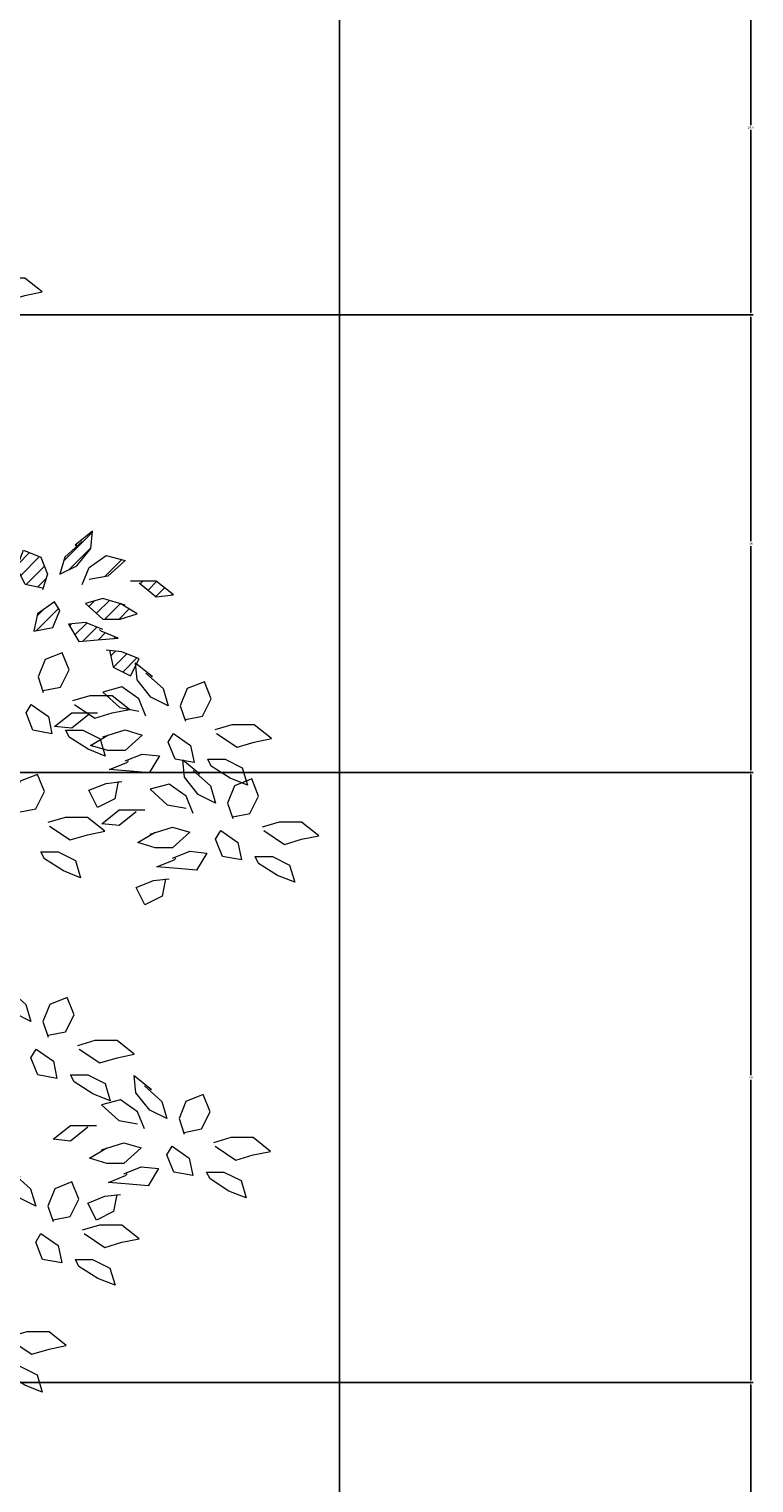
# Model space of a CAD drawing. Units: inches. Extents: x 1770 to 2988, y 1161 to 3221.
# Tile 43 of 44: x 2745 to 2802, y 2750 to 2865. Entities that reach past the tile are written whole.
import ezdxf

# ---------------------------------------------------------------- set-up
doc = ezdxf.new("R2010")
doc.units = ezdxf.units.IN
for name, color, linetype, lineweight in [('A-ANNO-DIMS', 2, 'Continuous', 18), ('A-ANNO-TTLB', 7, 'Continuous', 25), ('trees1', 250, 'Continuous', 13)]:
    doc.layers.add(name, color=color, linetype=linetype, lineweight=lineweight)
doc.styles.get("Standard").update_dxf_attribs({"font": 'arial.ttf'})
doc.dimstyles.get("Standard").update_dxf_attribs({"dimtxt": 0.18, "dimasz": 0.18, "dimexe": 0.18, "dimexo": 0.0625, "dimgap": 0.09, "dimtad": 0, "dimtih": 1, "dimtoh": 1, "dimdec": 4, "dimzin": 0, "dimdsep": 46, "dimtxsty": 'Standard', "dimcen": 0.09, "dimadec": 0, "dimazin": 0, "dimtfac": 1, "dimtdec": 4, "dimtofl": 0, "dimtmove": 0, "dimatfit": 3, "dimfxl": 1, "dimtolj": 1, "dimtzin": 0, "dimarcsym": 0})

# ---------------------------------------------------------------- blocks, each defined once
blk = doc.blocks.new('*X8')
at = {"color": 0}
for p, q in [((0.637, -0.8479), (0.6441, -0.8408)), ((0.6463, -0.8563), (0.6624, -0.8402)), ((0.6568, -0.8635), (0.676, -0.8443)), ((0.6745, -0.8635), (0.687, -0.8509))]:
    blk.add_line(p, q, dxfattribs=at)
blk = doc.blocks.new('*X6')
at = {"color": 0}
for p, q in [((0.6127, -0.8722), (0.6154, -0.8695)), ((0.6193, -0.8833), (0.6342, -0.8684)), ((0.6293, -0.8909), (0.6469, -0.8734)), ((0.6488, -0.8892), (0.6573, -0.8806)), ((0.6681, -0.8876), (0.67, -0.8857))]:
    blk.add_line(p, q, dxfattribs=at)
blk = doc.blocks.new('*X14')
at = {"color": 0}
blk.add_line((0.6567, -0.8106), (0.6779, -0.7894), dxfattribs=at)
blk = doc.blocks.new('*X11')
at = {"color": 0}
for p, q in [((0.5716, -0.8779), (0.5992, -0.8504)), ((0.5721, -0.8598), (0.5799, -0.852))]:
    blk.add_line(p, q, dxfattribs=at)
blk = doc.blocks.new('*X15')
at = {"color": 0}
for p, q in [((0.6056, -0.7909), (0.6413, -0.7553)), ((0.6124, -0.8018), (0.6393, -0.7749))]:
    blk.add_line(p, q, dxfattribs=at)
blk = doc.blocks.new('*X9')
at = {"color": 0}
for p, q in [((0.7007, -0.8195), (0.704, -0.8163)), ((0.7106, -0.8274), (0.7213, -0.8167)), ((0.7204, -0.8352), (0.7311, -0.8245)), ((0.7396, -0.8337), (0.7409, -0.8324))]:
    blk.add_line(p, q, dxfattribs=at)
blk = doc.blocks.new('*X13')
at = {"color": 0}
for p, q in [((0.5486, -0.7949), (0.5629, -0.7806)), ((0.552, -0.8092), (0.5755, -0.7857)), ((0.5582, -0.8207), (0.5814, -0.7974)), ((0.5729, -0.8236), (0.5839, -0.8126))]:
    blk.add_line(p, q, dxfattribs=at)
blk = doc.blocks.new('*X7')
at = {"color": 0}
for p, q in [((0.6642, -0.9091), (0.6699, -0.9034)), ((0.6673, -0.9237), (0.6842, -0.9068)), ((0.6791, -0.9296), (0.6968, -0.9118))]:
    blk.add_line(p, q, dxfattribs=at)
blk = doc.blocks.new('tree342')
at = {"color": 0}
for points in [[(352.8, 2116), (378.6, 2098.8), (400, 2105.2), (421.5, 2109.5), (400, 2126.7), (372.1, 2126.7), (350.6, 2120.2)], [(471.5, 1798.5), (450, 1779.2), (443.6, 1757.7), (465, 1768.4), (482.2, 1789.9), (484.4, 1811.3), (462.9, 1794.2), (465, 1794.2)], [(422.1, 1740.5), (400.6, 1744.8), (389.9, 1766.3), (398.5, 1787.7), (420, 1779.2), (428.5, 1757.7), (422.1, 1738.4)], [(471.5, 1744.8), (480.1, 1766.3), (501.6, 1781.3), (525.2, 1774.9), (503.7, 1755.5), (480.1, 1751.3)], [(542.4, 1747), (563.8, 1729.8), (585.3, 1731.9), (563.8, 1749.1), (531.6, 1749.1)], [(525.2, 1719.1), (497.3, 1727.6), (475.8, 1721.2), (497.3, 1701.9), (518.7, 1701.9), (540.2, 1708.3), (518.7, 1721.2)], [(497.3, 1689), (475.8, 1697.6), (454.3, 1695.5), (467.2, 1674), (490.8, 1676.1), (516.6, 1678.3), (495.1, 1686.9), (493, 1689)], [(423.1, 1612.8), (444.6, 1617.1), (455.3, 1638.5), (446.7, 1660), (425.3, 1651.4), (416.7, 1629.9), (423.1, 1610.6)], [(505.8, 1663.3), (510.1, 1641.8), (531.6, 1631.1), (542.4, 1652.5), (520.9, 1661.1), (501.6, 1663.3)], [(550.8, 1634.6), (572.3, 1615.2), (578.8, 1593.8), (557.3, 1604.5), (540.1, 1626), (538, 1647.4), (559.4, 1630.3), (557.3, 1630.3)], [(550.8, 1580.9), (542.2, 1602.4), (520.8, 1617.4), (497.2, 1611), (518.6, 1591.6), (542.2, 1587.3)], [(600.2, 1576.6), (621.7, 1580.9), (632.4, 1602.4), (623.9, 1623.8), (602.4, 1615.2), (593.8, 1593.8), (600.2, 1574.5)], [(461.8, 1595.6), (487.5, 1578.4), (509, 1584.9), (530.5, 1589.2), (509, 1606.3), (481.1, 1606.3), (459.6, 1599.9)], [(480, 1583.1), (458.5, 1565.9), (437, 1568), (458.5, 1585.2), (490.7, 1585.2)], [(497.2, 1555.2), (525.1, 1563.7), (546.5, 1557.3), (525.1, 1538), (503.6, 1538), (482.1, 1544.4), (503.6, 1557.3)], [(638.9, 1559.5), (664.7, 1542.3), (686.1, 1548.7), (707.6, 1553), (686.1, 1570.2), (658.2, 1570.2), (636.7, 1563.7)], [(525.1, 1525.1), (546.5, 1533.7), (568, 1531.6), (555.1, 1510.1), (531.5, 1512.2), (505.7, 1514.4), (527.2, 1523), (529.4, 1525.1)], [(609.9, 1513.4), (631.3, 1494.1), (637.8, 1472.6), (616.3, 1483.4), (599.1, 1504.8), (597, 1526.3), (618.4, 1509.1), (616.3, 1509.1)], [(392.2, 1461.1), (413.7, 1465.4), (424.4, 1486.9), (415.9, 1508.4), (394.4, 1499.8), (385.8, 1478.3), (392.2, 1459)], [(516.5, 1499.4), (512.2, 1477.9), (490.7, 1467.2), (480, 1488.6), (501.4, 1497.2), (520.8, 1499.4)], [(609.9, 1459.8), (601.3, 1481.2), (579.8, 1496.2), (556.2, 1489.8), (577.6, 1470.5), (601.3, 1466.2)], [(659.2, 1455.5), (680.7, 1459.8), (691.5, 1481.2), (682.9, 1502.7), (661.4, 1494.1), (652.8, 1472.6), (659.2, 1453.3)], [(430.9, 1444), (456.7, 1426.8), (478.1, 1433.2), (499.6, 1437.5), (478.1, 1454.7), (450.2, 1454.7), (428.7, 1448.3)], [(539, 1461.9), (517.5, 1444.7), (496, 1446.9), (517.5, 1464.1), (549.7, 1464.1)], [(556.2, 1434), (584.1, 1442.6), (605.6, 1436.2), (584.1, 1416.8), (562.6, 1416.8), (541.1, 1423.3), (562.6, 1436.2)], [(697.9, 1438.3), (723.7, 1421.1), (745.1, 1427.6), (766.6, 1431.9), (745.1, 1449), (717.2, 1449), (695.8, 1442.6)], [(584.1, 1404), (605.6, 1412.5), (627, 1410.4), (614.1, 1388.9), (590.5, 1391.1), (564.8, 1393.2), (586.2, 1401.8), (588.4, 1404)], [(575.5, 1378.2), (571.2, 1356.8), (549.7, 1346), (539, 1367.5), (560.5, 1376.1), (579.8, 1378.2)], [(379.8, 1241.1), (401.3, 1221.8), (407.7, 1200.4), (386.2, 1211.1), (369, 1232.6), (366.9, 1254), (388.4, 1236.8), (386.2, 1236.8)], [(429.2, 1183.2), (450.6, 1187.5), (461.4, 1208.9), (452.8, 1230.4), (431.3, 1221.8), (422.7, 1200.4), (429.2, 1181)], [(467.8, 1166), (493.6, 1148.9), (515.1, 1155.3), (536.5, 1159.6), (515.1, 1176.8), (487.2, 1176.8), (465.7, 1170.3)], [(549.3, 1120.1), (570.8, 1100.8), (577.2, 1079.4), (555.8, 1090.1), (538.6, 1111.5), (536.4, 1133), (557.9, 1115.8), (555.8, 1115.8)], [(598.7, 1062.2), (620.2, 1066.5), (630.9, 1087.9), (622.3, 1109.4), (600.8, 1100.8), (592.3, 1079.4), (598.7, 1060)], [(549.3, 1066.5), (540.7, 1087.9), (519.2, 1103), (495.6, 1096.5), (517.1, 1077.2), (540.7, 1072.9)], [(478.4, 1068.6), (457, 1051.5), (435.5, 1053.6), (457, 1070.8), (489.2, 1070.8)], [(637.4, 1045), (663.1, 1027.8), (684.6, 1034.3), (706.1, 1038.6), (684.6, 1055.7), (656.7, 1055.7), (635.2, 1049.3)], [(495.6, 1040.7), (523.5, 1049.3), (545, 1042.9), (523.5, 1023.6), (502.1, 1023.6), (480.6, 1030), (502.1, 1042.9)], [(385.8, 1011.2), (407.3, 991.9), (413.8, 970.4), (392.3, 981.2), (375.1, 1002.6), (373, 1024.1), (394.4, 1006.9), (392.3, 1006.9)], [(523.5, 1010.7), (545, 1019.3), (566.5, 1017.1), (553.6, 995.7), (530, 997.8), (504.2, 999.9), (525.7, 1008.5), (527.8, 1010.7)], [(435.2, 953.3), (456.7, 957.6), (467.4, 979), (458.8, 1000.5), (437.4, 991.9), (428.8, 970.4), (435.2, 951.1)], [(514.9, 984.9), (510.7, 963.5), (489.2, 952.7), (478.4, 974.2), (499.9, 982.8), (519.2, 984.9)], [(473.9, 936.1), (499.6, 918.9), (521.1, 925.4), (542.6, 929.7), (521.1, 946.8), (493.2, 946.8), (471.7, 940.4)], [(383.1, 803), (408.8, 785.8), (430.3, 792.3), (451.8, 796.6), (430.3, 813.7), (402.4, 813.7), (380.9, 807.3)]]:
    blk.add_lwpolyline(points, dxfattribs=at)
for points in [[(415.7, 1708.3), (411.4, 1686.9), (435, 1691.2), (443.6, 1712.6), (437.1, 1723.4)], [(429.6, 1580.6), (433.9, 1559.1), (410.2, 1563.4), (401.6, 1584.9), (408.1, 1595.6)], [(472.5, 1563.4), (494, 1552.7), (500.4, 1531.2), (479, 1539.8), (455.3, 1554.8), (451, 1563.4)], [(606.7, 1544.4), (611, 1523), (587.3, 1527.3), (578.8, 1548.7), (585.2, 1559.5)], [(649.6, 1527.3), (671.1, 1516.5), (677.5, 1495.1), (656.1, 1503.7), (632.4, 1518.7), (628.1, 1527.3)], [(665.7, 1423.3), (670, 1401.8), (646.4, 1406.1), (637.8, 1427.6), (644.2, 1438.3)], [(441.6, 1411.8), (463.1, 1401.1), (469.5, 1379.6), (448.1, 1388.2), (424.4, 1403.2), (420.1, 1411.8)], [(708.6, 1406.1), (730.1, 1395.4), (736.6, 1373.9), (715.1, 1382.5), (691.5, 1397.5), (687.2, 1406.1)], [(435.6, 1151), (439.9, 1129.5), (416.3, 1133.8), (407.7, 1155.3), (414.1, 1166)], [(478.6, 1133.8), (500, 1123.1), (506.5, 1101.6), (485, 1110.2), (461.4, 1125.3), (457.1, 1133.8)], [(605.1, 1030), (609.4, 1008.5), (585.8, 1012.8), (577.2, 1034.3), (583.7, 1045)], [(648.1, 1012.8), (669.6, 1002.1), (676, 980.6), (654.5, 989.2), (630.9, 1004.2), (626.6, 1012.8)], [(441.7, 921.1), (446, 899.6), (422.3, 903.9), (413.8, 925.4), (420.2, 936.1)], [(484.6, 903.9), (506.1, 893.2), (512.5, 871.7), (491.1, 880.3), (467.4, 895.3), (463.1, 903.9)], [(393.8, 770.8), (415.3, 760.1), (421.7, 738.6), (400.2, 747.2), (376.6, 762.2), (372.3, 770.8)]]:
    blk.add_lwpolyline(points, close=True, dxfattribs=at)
at = {"color": 0, "xscale": 1000, "yscale": 1000, "zscale": 1000}
for name in ['*X15', '*X13', '*X14', '*X9', '*X8', '*X11', '*X6', '*X7']:
    blk.add_blockref(name, (-157, 2565.4), dxfattribs=at)
blk = doc.blocks.new('*D96')
at = {"layer": 'A-ANNO-DIMS', "color": 0, "lineweight": -2, "transparency": 16777216}
for p, q in [((2620.11, 2758.3), (2801.91, 2758.3)), ((2801.73, 2758.12), (2801.73, 2740.48)), ((2801.73, 2722.48), (2801.73, 2740.11)), ((2655.51, 2722.3), (2801.91, 2722.3))]:
    blk.add_line(p, q, dxfattribs=at)
at = {"layer": 'A-ANNO-DIMS', "color": 0, "transparency": 16777216}
for points in [[(2801.7, 2758.12), (2801.76, 2758.12), (2801.73, 2758.3)], [(2801.7, 2722.48), (2801.76, 2722.48), (2801.73, 2722.3)]]:
    blk.add_solid(points, dxfattribs=at)
at = {"layer": 'Defpoints', "color": 0, "transparency": 16777216}
for p in [(2620.05, 2758.3), (2801.73, 2758.3), (2655.44, 2722.3)]:
    blk.add_point(p, dxfattribs=at)
at = {"layer": 'A-ANNO-DIMS', "color": 0, "transparency": 16777216, "insert": (2801.73, 2740.3), "char_height": 0.18, "attachment_point": 5}
blk.add_mtext('\\A1;36', dxfattribs=at)
blk = doc.blocks.new('*D97')
at = {"layer": 'A-ANNO-DIMS', "color": 0, "lineweight": -2, "transparency": 16777216}
for p, q in [((2620.11, 2806.3), (2801.91, 2806.3)), ((2801.73, 2806.12), (2801.73, 2782.48)), ((2801.73, 2758.48), (2801.73, 2782.11)), ((2620.11, 2758.3), (2801.91, 2758.3))]:
    blk.add_line(p, q, dxfattribs=at)
at = {"layer": 'A-ANNO-DIMS', "color": 0, "transparency": 16777216}
for points in [[(2801.7, 2806.12), (2801.76, 2806.12), (2801.73, 2806.3)], [(2801.7, 2758.48), (2801.76, 2758.48), (2801.73, 2758.3)]]:
    blk.add_solid(points, dxfattribs=at)
at = {"layer": 'Defpoints', "color": 0, "transparency": 16777216}
for p in [(2620.05, 2806.3), (2801.73, 2806.3), (2620.05, 2758.3)]:
    blk.add_point(p, dxfattribs=at)
at = {"layer": 'A-ANNO-DIMS', "color": 0, "transparency": 16777216, "insert": (2801.73, 2782.3), "char_height": 0.18, "attachment_point": 5}
blk.add_mtext('\\A1;48', dxfattribs=at)
blk = doc.blocks.new('*D98')
at = {"layer": 'A-ANNO-DIMS', "color": 0, "lineweight": -2, "transparency": 16777216}
for p, q in [((2655.51, 2842.3), (2801.91, 2842.3)), ((2801.73, 2842.12), (2801.73, 2824.48)), ((2801.73, 2806.48), (2801.73, 2824.11)), ((2620.11, 2806.3), (2801.91, 2806.3))]:
    blk.add_line(p, q, dxfattribs=at)
at = {"layer": 'A-ANNO-DIMS', "color": 0, "transparency": 16777216}
for points in [[(2801.7, 2842.12), (2801.76, 2842.12), (2801.73, 2842.3)], [(2801.7, 2806.48), (2801.76, 2806.48), (2801.73, 2806.3)]]:
    blk.add_solid(points, dxfattribs=at)
at = {"layer": 'Defpoints', "color": 0, "transparency": 16777216}
for p in [(2655.44, 2842.3), (2801.73, 2842.3), (2620.05, 2806.3)]:
    blk.add_point(p, dxfattribs=at)
at = {"layer": 'A-ANNO-DIMS', "color": 0, "transparency": 16777216, "insert": (2801.73, 2824.3), "char_height": 0.18, "attachment_point": 5}
blk.add_mtext('\\A1;36', dxfattribs=at)
blk = doc.blocks.new('*D99')
at = {"layer": 'A-ANNO-DIMS', "color": 0, "lineweight": -2, "transparency": 16777216}
for p, q in [((2655.51, 2871.79), (2801.91, 2871.79)), ((2801.73, 2871.61), (2801.73, 2857.23)), ((2801.73, 2842.48), (2801.73, 2856.86)), ((2655.51, 2842.3), (2801.91, 2842.3))]:
    blk.add_line(p, q, dxfattribs=at)
at = {"layer": 'A-ANNO-DIMS', "color": 0, "transparency": 16777216}
for points in [[(2801.7, 2871.61), (2801.76, 2871.61), (2801.73, 2871.79)], [(2801.7, 2842.48), (2801.76, 2842.48), (2801.73, 2842.3)]]:
    blk.add_solid(points, dxfattribs=at)
at = {"layer": 'Defpoints', "color": 0, "transparency": 16777216}
for p in [(2655.44, 2871.79), (2801.73, 2871.79), (2655.44, 2842.3)]:
    blk.add_point(p, dxfattribs=at)
at = {"layer": 'A-ANNO-DIMS', "color": 0, "transparency": 16777216, "insert": (2801.73, 2857.05), "char_height": 0.18, "attachment_point": 5}
blk.add_mtext('\\A1;29.5', dxfattribs=at)

msp = doc.modelspace()

# ---------------------------------------------------------------- linework, layer by layer
at = {"layer": 'A-ANNO-TTLB'}
msp.add_lwpolyline([(2073.6202, 3129.9468), (2769.3644, 3129.9468), (2769.3644, 2546.8952), (2073.6202, 2546.8952)], close=True, dxfattribs=at)

# ---------------------------------------------------------------- block references
at = {"layer": 'trees1', "xscale": 0.063143750371755, "yscale": 0.063143750371755, "zscale": 0.063143750371755}
msp.add_blockref('tree342', (2719.3275, 2710.8976), dxfattribs=at)

# ---------------------------------------------------------------- dimensions: what is measured, and where the dimension line sits
at = {"layer": 'A-ANNO-DIMS'}
for base, p1, p2, override, picture, middle in [((2801.7346, 2871.7944), (2655.443, 2842.2969), (2655.443, 2871.7944), {"dimdec": 1, "dimlfac": 1, "dimrnd": 0, "dimzin": 0, "dimdsep": 46, "dimlunit": 2}, '*D99', (2801.7346, 2857.0456)), ((2801.7346, 2842.2969), (2620.0508, 2806.2969), (2655.443, 2842.2969), {"dimdec": 0, "dimlfac": 1, "dimrnd": 0, "dimzin": 0, "dimdsep": 46, "dimlunit": 2}, '*D98', (2801.7346, 2824.2969)), ((2801.7346, 2806.2969), (2620.0508, 2758.2969), (2620.0508, 2806.2969), {"dimdec": 0, "dimlfac": 1, "dimrnd": 0, "dimzin": 0, "dimdsep": 46, "dimlunit": 2}, '*D97', (2801.7346, 2782.2969)), ((2801.7346, 2758.2969), (2655.443, 2722.2969), (2620.0508, 2758.2969), {"dimdec": 0, "dimlfac": 1, "dimrnd": 0, "dimzin": 0, "dimdsep": 46, "dimlunit": 2}, '*D96', (2801.7346, 2740.2969))]:
    dim = msp.add_linear_dim(base=base, p1=p1, p2=p2, angle=90, dimstyle='Standard', override=override, dxfattribs=at)
    dim.commit()
    dim.dimension.update_dxf_attribs({"geometry": picture, "text_midpoint": middle})

doc.saveas('drawing.dxf')
